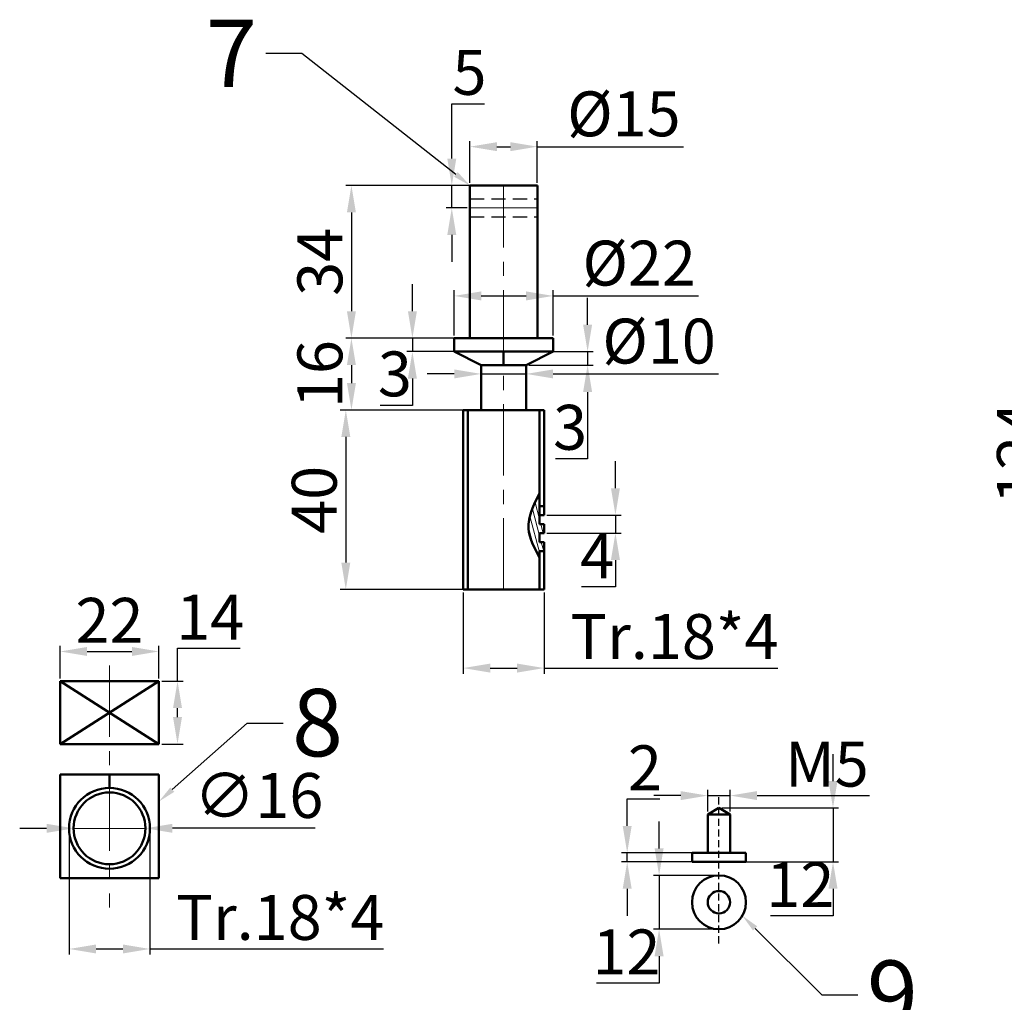
# Model space of a CAD drawing. Units: millimetres. Extents: x 147 to 984, y -369 to 435.
# Tile 6 of 10: x 480 to 699, y -48 to 171. Entities that reach past the tile are written whole.
import ezdxf
from ezdxf import colors
from ezdxf.entities.mleader import LeaderData, LeaderLine
from ezdxf.math import Vec2, Vec3

# ---------------------------------------------------------------- set-up
doc = ezdxf.new("R2010")
doc.units = ezdxf.units.MM
doc.header["$LTSCALE"] = 0.5
doc.linetypes.add('CENTER', pattern=[50.8, 31.75, -6.35, 6.35, -6.35])
doc.linetypes.add('HIDDEN', pattern=[9.525, 6.35, -3.175])
for name, color, linetype, lineweight in [('M-CNTR', 1, 'CENTER', 18), ('M-DIMS', 2, 'Continuous', 25), ('M-HATC', 8, 'Continuous', 18), ('M-HIDN', 3, 'HIDDEN', 25), ('M-OUTL', 7, 'Continuous', 50), ('M-TEXT', 7, 'Continuous', 25)]:
    doc.layers.add(name, color=color, linetype=linetype, lineweight=lineweight)
doc.styles.get("Standard").update_dxf_attribs({"font": 'arial.ttf'})
doc.dimstyles.new('ISO-25', dxfattribs={"dimtxt": 10, "dimasz": 6, "dimexe": 1.25, "dimexo": 0.625, "dimtad": 1, "dimtoh": 1, "dimdec": 0, "dimtxsty": 'Standard', "dimcen": 2.5, "dimadec": 0, "dimazin": 0, "dimtfac": 1, "dimtdec": 0, "dimtmove": 0, "dimatfit": 3, "dimfxl": 1, "dimarcsym": 0})

# ---------------------------------------------------------------- blocks, each defined once
blk = doc.blocks.new('*D63')
at = {"layer": 'Defpoints', "color": 0, "transparency": 16777216}
for p in [(800.56, 136.03), (709.78, 12.03), (800.56, 12.03)]:
    blk.add_point(p, dxfattribs=at)
at = {"layer": 'M-DIMS', "color": 0, "lineweight": -2, "transparency": 16777216}
for p, q in [((799.93, 136.03), (708.53, 136.03)), ((709.78, 130.03), (709.78, 18.03)), ((799.93, 12.03), (708.53, 12.03))]:
    blk.add_line(p, q, dxfattribs=at)
at = {"layer": 'M-DIMS', "color": 0, "transparency": 16777216}
for points in [[(708.78, 130.03), (710.78, 130.03), (709.78, 136.03)], [(708.78, 18.03), (710.78, 18.03), (709.78, 12.03)]]:
    blk.add_solid(points, dxfattribs=at)
at = {"layer": 'M-DIMS', "color": 0, "transparency": 16777216, "insert": (704.14, 74.03), "char_height": 10, "attachment_point": 5, "rotation": 90}
blk.add_mtext('124', dxfattribs=at)
blk = doc.blocks.new('*D75')
at = {"layer": 'Defpoints', "color": 0, "ltscale": 0.5, "transparency": 16777216}
for p in [(595.48, 142.24), (580.48, 133.59), (595.48, 133.59)]:
    blk.add_point(p, dxfattribs=at)
at = {"layer": 'M-DIMS', "color": 0, "lineweight": -2, "ltscale": 0.5, "transparency": 16777216}
for p, q in [((580.48, 134.22), (580.48, 143.49)), ((595.48, 134.22), (595.48, 143.49)), ((586.48, 142.24), (589.48, 142.24)), ((595.48, 142.24), (628.01, 142.24))]:
    blk.add_line(p, q, dxfattribs=at)
at = {"layer": 'M-DIMS', "color": 0, "ltscale": 0.5, "transparency": 16777216}
for points in [[(586.48, 143.24), (586.48, 141.24), (580.48, 142.24)], [(589.48, 143.24), (589.48, 141.24), (595.48, 142.24)]]:
    blk.add_solid(points, dxfattribs=at)
at = {"layer": 'M-DIMS', "color": 0, "ltscale": 0.5, "transparency": 16777216, "insert": (614.75, 148.25), "char_height": 10, "attachment_point": 5}
blk.add_mtext('%%C15', dxfattribs=at)
blk = doc.blocks.new('*D76')
at = {"layer": 'Defpoints', "color": 0, "ltscale": 0.5, "transparency": 16777216}
for p in [(580.48, 133.59), (576.43, 128.59), (580.48, 128.59)]:
    blk.add_point(p, dxfattribs=at)
at = {"layer": 'M-DIMS', "color": 0, "lineweight": -2, "ltscale": 0.5, "transparency": 16777216}
for p, q in [((576.43, 139.59), (576.43, 151.78)), ((576.43, 151.78), (583.68, 151.78)), ((579.86, 133.59), (575.18, 133.59)), ((576.43, 128.59), (576.43, 133.59)), ((579.86, 128.59), (575.18, 128.59)), ((576.43, 122.59), (576.43, 116.59))]:
    blk.add_line(p, q, dxfattribs=at)
at = {"layer": 'M-DIMS', "color": 0, "ltscale": 0.5, "transparency": 16777216}
for points in [[(575.43, 139.59), (577.43, 139.59), (576.43, 133.59)], [(575.43, 122.59), (577.43, 122.59), (576.43, 128.59)]]:
    blk.add_solid(points, dxfattribs=at)
at = {"layer": 'M-DIMS', "color": 0, "ltscale": 0.5, "transparency": 16777216, "insert": (580.37, 157.49), "char_height": 10, "attachment_point": 5}
blk.add_mtext('5', dxfattribs=at)
blk = doc.blocks.new('*D77')
at = {"layer": 'Defpoints', "color": 0, "ltscale": 0.5, "transparency": 16777216}
for p in [(587.98, 133.59), (554.08, 99.59), (587.98, 99.59)]:
    blk.add_point(p, dxfattribs=at)
at = {"layer": 'M-DIMS', "color": 0, "lineweight": -2, "ltscale": 0.5, "transparency": 16777216}
for p, q in [((587.36, 133.59), (552.83, 133.59)), ((554.08, 127.59), (554.08, 105.59)), ((587.36, 99.59), (552.83, 99.59))]:
    blk.add_line(p, q, dxfattribs=at)
at = {"layer": 'M-DIMS', "color": 0, "ltscale": 0.5, "transparency": 16777216}
for points in [[(553.08, 127.59), (555.08, 127.59), (554.08, 133.59)], [(553.08, 105.59), (555.08, 105.59), (554.08, 99.59)]]:
    blk.add_solid(points, dxfattribs=at)
at = {"layer": 'M-DIMS', "color": 0, "ltscale": 0.5, "transparency": 16777216, "insert": (548.35, 116.59), "char_height": 10, "attachment_point": 5, "rotation": 90}
blk.add_mtext('34', dxfattribs=at)
blk = doc.blocks.new('*D78')
at = {"layer": 'Defpoints', "color": 0, "ltscale": 0.5, "transparency": 16777216}
for p in [(587.98, 99.59), (554.08, 83.59), (587.98, 83.59)]:
    blk.add_point(p, dxfattribs=at)
at = {"layer": 'M-DIMS', "color": 0, "lineweight": -2, "ltscale": 0.5, "transparency": 16777216}
for p, q in [((587.36, 99.59), (552.83, 99.59)), ((554.08, 93.59), (554.08, 89.59)), ((587.36, 83.59), (552.83, 83.59))]:
    blk.add_line(p, q, dxfattribs=at)
at = {"layer": 'M-DIMS', "color": 0, "ltscale": 0.5, "transparency": 16777216}
for points in [[(553.08, 93.59), (555.08, 93.59), (554.08, 99.59)], [(553.08, 89.59), (555.08, 89.59), (554.08, 83.59)]]:
    blk.add_solid(points, dxfattribs=at)
at = {"layer": 'M-DIMS', "color": 0, "ltscale": 0.5, "transparency": 16777216, "insert": (548.35, 91.59), "char_height": 10, "attachment_point": 5, "rotation": 90}
blk.add_mtext('16', dxfattribs=at)
blk = doc.blocks.new('*D79')
at = {"layer": 'Defpoints', "color": 0, "ltscale": 0.5, "transparency": 16777216}
for p in [(587.98, 83.59), (552.83, 43.59), (587.98, 43.59)]:
    blk.add_point(p, dxfattribs=at)
at = {"layer": 'M-DIMS', "color": 0, "lineweight": -2, "ltscale": 0.5, "transparency": 16777216}
for p, q in [((587.36, 83.59), (551.58, 83.59)), ((552.83, 77.59), (552.83, 49.59)), ((587.36, 43.59), (551.58, 43.59))]:
    blk.add_line(p, q, dxfattribs=at)
at = {"layer": 'M-DIMS', "color": 0, "ltscale": 0.5, "transparency": 16777216}
for points in [[(551.83, 77.59), (553.83, 77.59), (552.83, 83.59)], [(551.83, 49.59), (553.83, 49.59), (552.83, 43.59)]]:
    blk.add_solid(points, dxfattribs=at)
at = {"layer": 'M-DIMS', "color": 0, "ltscale": 0.5, "transparency": 16777216, "insert": (547.1, 63.59), "char_height": 10, "attachment_point": 5, "rotation": 90}
blk.add_mtext('40', dxfattribs=at)
blk = doc.blocks.new('*D80')
at = {"layer": 'Defpoints', "color": 0, "ltscale": 0.5, "transparency": 16777216}
for p in [(592.98, 91.63), (582.98, 88.59), (592.98, 88.59)]:
    blk.add_point(p, dxfattribs=at)
at = {"layer": 'M-DIMS', "color": 0, "lineweight": -2, "ltscale": 0.5, "transparency": 16777216}
for p, q in [((582.98, 89.22), (582.98, 92.88)), ((592.98, 89.22), (592.98, 92.88)), ((576.98, 91.63), (570.98, 91.63)), ((582.98, 91.63), (592.98, 91.63)), ((598.98, 91.63), (635.81, 91.63))]:
    blk.add_line(p, q, dxfattribs=at)
at = {"layer": 'M-DIMS', "color": 0, "ltscale": 0.5, "transparency": 16777216}
for points in [[(576.98, 92.63), (576.98, 90.63), (582.98, 91.63)], [(598.98, 92.63), (598.98, 90.63), (592.98, 91.63)]]:
    blk.add_solid(points, dxfattribs=at)
at = {"layer": 'M-DIMS', "color": 0, "ltscale": 0.5, "transparency": 16777216, "insert": (622.6, 97.64), "char_height": 10, "attachment_point": 5}
blk.add_mtext('%%C10', dxfattribs=at)
blk = doc.blocks.new('*D81')
at = {"layer": 'Defpoints', "color": 0, "ltscale": 0.5, "transparency": 16777216}
for p in [(598.98, 109), (576.98, 99.59), (598.98, 99.59)]:
    blk.add_point(p, dxfattribs=at)
at = {"layer": 'M-DIMS', "color": 0, "lineweight": -2, "ltscale": 0.5, "transparency": 16777216}
for p, q in [((576.98, 100.22), (576.98, 110.25)), ((598.98, 100.22), (598.98, 110.25)), ((582.98, 109), (592.98, 109)), ((598.98, 109), (631.34, 109))]:
    blk.add_line(p, q, dxfattribs=at)
at = {"layer": 'M-DIMS', "color": 0, "ltscale": 0.5, "transparency": 16777216}
for points in [[(582.98, 110), (582.98, 108), (576.98, 109)], [(592.98, 110), (592.98, 108), (598.98, 109)]]:
    blk.add_solid(points, dxfattribs=at)
at = {"layer": 'M-DIMS', "color": 0, "ltscale": 0.5, "transparency": 16777216, "insert": (618.16, 115.01), "char_height": 10, "attachment_point": 5}
blk.add_mtext('%%C22', dxfattribs=at)
blk = doc.blocks.new('*D82')
at = {"layer": 'Defpoints', "color": 0, "ltscale": 0.5, "transparency": 16777216}
for p in [(587.98, 99.59), (567.66, 96.59), (587.98, 96.59)]:
    blk.add_point(p, dxfattribs=at)
at = {"layer": 'M-DIMS', "color": 0, "lineweight": -2, "ltscale": 0.5, "transparency": 16777216}
for p, q in [((567.66, 105.59), (567.66, 111.59)), ((587.36, 99.59), (566.41, 99.59)), ((567.66, 99.59), (567.66, 96.59)), ((587.36, 96.59), (566.41, 96.59)), ((567.66, 90.59), (567.66, 84.59)), ((567.66, 84.59), (560.49, 84.59))]:
    blk.add_line(p, q, dxfattribs=at)
at = {"layer": 'M-DIMS', "color": 0, "ltscale": 0.5, "transparency": 16777216}
for points in [[(566.66, 105.59), (568.66, 105.59), (567.66, 99.59)], [(566.66, 90.59), (568.66, 90.59), (567.66, 96.59)]]:
    blk.add_solid(points, dxfattribs=at)
at = {"layer": 'M-DIMS', "color": 0, "ltscale": 0.5, "transparency": 16777216, "insert": (563.76, 90.33), "char_height": 10, "attachment_point": 5}
blk.add_mtext('3', dxfattribs=at)
blk = doc.blocks.new('*D83')
at = {"layer": 'Defpoints', "color": 0, "ltscale": 0.5, "transparency": 16777216}
for p in [(592.98, 96.59), (606.68, 96.59), (592.98, 93.59)]:
    blk.add_point(p, dxfattribs=at)
at = {"layer": 'M-DIMS', "color": 0, "lineweight": -2, "ltscale": 0.5, "transparency": 16777216}
for p, q in [((606.68, 102.59), (606.68, 108.59)), ((593.61, 96.59), (607.93, 96.59)), ((606.68, 96.59), (606.68, 93.59)), ((593.61, 93.59), (607.93, 93.59)), ((606.68, 87.59), (606.68, 72.7)), ((606.68, 72.7), (599.5, 72.7))]:
    blk.add_line(p, q, dxfattribs=at)
at = {"layer": 'M-DIMS', "color": 0, "ltscale": 0.5, "transparency": 16777216}
for points in [[(605.68, 102.59), (607.68, 102.59), (606.68, 96.59)], [(605.68, 87.59), (607.68, 87.59), (606.68, 93.59)]]:
    blk.add_solid(points, dxfattribs=at)
at = {"layer": 'M-DIMS', "color": 0, "ltscale": 0.5, "transparency": 16777216, "insert": (602.78, 78.44), "char_height": 10, "attachment_point": 5}
blk.add_mtext('3', dxfattribs=at)
blk = doc.blocks.new('*D84')
at = {"layer": 'Defpoints', "color": 0, "ltscale": 0.5, "transparency": 16777216}
for p in [(596.98, 60.18), (596.98, 56.18), (612.88, 56.18)]:
    blk.add_point(p, dxfattribs=at)
at = {"layer": 'M-DIMS', "color": 0, "lineweight": -2, "ltscale": 0.5, "transparency": 16777216}
for p, q in [((612.88, 66.18), (612.88, 72.18)), ((597.61, 60.18), (614.13, 60.18)), ((612.88, 60.18), (612.88, 56.18)), ((597.61, 56.18), (614.13, 56.18)), ((612.88, 50.18), (612.88, 44.18)), ((612.88, 44.18), (605.34, 44.18))]:
    blk.add_line(p, q, dxfattribs=at)
at = {"layer": 'M-DIMS', "color": 0, "ltscale": 0.5, "transparency": 16777216}
for points in [[(611.88, 66.18), (613.88, 66.18), (612.88, 60.18)], [(611.88, 50.18), (613.88, 50.18), (612.88, 56.18)]]:
    blk.add_solid(points, dxfattribs=at)
at = {"layer": 'M-DIMS', "color": 0, "ltscale": 0.5, "transparency": 16777216, "insert": (608.8, 49.81), "char_height": 10, "attachment_point": 5}
blk.add_mtext('4', dxfattribs=at)
blk = doc.blocks.new('*D85')
at = {"layer": 'Defpoints', "color": 0, "ltscale": 0.5, "transparency": 16777216}
for p in [(578.98, 43.59), (596.98, 43.59), (596.98, 26.11)]:
    blk.add_point(p, dxfattribs=at)
at = {"layer": 'M-DIMS', "color": 0, "lineweight": -2, "ltscale": 0.5, "transparency": 16777216}
for p, q in [((578.98, 42.97), (578.98, 24.86)), ((596.98, 42.97), (596.98, 24.86)), ((584.98, 26.11), (590.98, 26.11)), ((596.98, 26.11), (649.04, 26.11))]:
    blk.add_line(p, q, dxfattribs=at)
at = {"layer": 'M-DIMS', "color": 0, "ltscale": 0.5, "transparency": 16777216}
for points in [[(584.98, 27.11), (584.98, 25.11), (578.98, 26.11)], [(590.98, 27.11), (590.98, 25.11), (596.98, 26.11)]]:
    blk.add_solid(points, dxfattribs=at)
at = {"layer": 'M-DIMS', "color": 0, "ltscale": 0.5, "transparency": 16777216, "insert": (626.01, 31.84), "char_height": 10, "attachment_point": 5}
blk.add_mtext('Tr.18*4', dxfattribs=at)
blk = doc.blocks.new('*U86')
at = {"layer": 'M-CNTR', "color": 0, "transparency": 16777216}
blk.add_line((0, 10.5), (0, -43.39), dxfattribs=at)
blk = doc.blocks.new('*D87')
at = {"layer": 'Defpoints', "color": 0, "ltscale": 0.5, "transparency": 16777216}
for p in [(491.2, -9.58), (509.2, -9.58), (509.2, -36.45)]:
    blk.add_point(p, dxfattribs=at)
at = {"layer": 'M-DIMS', "color": 0, "lineweight": -2, "ltscale": 0.5, "transparency": 16777216}
for p, q in [((491.2, -10.2), (491.2, -37.7)), ((509.2, -10.2), (509.2, -37.7)), ((497.2, -36.45), (503.2, -36.45)), ((509.2, -36.45), (561.26, -36.45))]:
    blk.add_line(p, q, dxfattribs=at)
at = {"layer": 'M-DIMS', "color": 0, "ltscale": 0.5, "transparency": 16777216}
for points in [[(497.2, -35.45), (497.2, -37.45), (491.2, -36.45)], [(503.2, -35.45), (503.2, -37.45), (509.2, -36.45)]]:
    blk.add_solid(points, dxfattribs=at)
at = {"layer": 'M-DIMS', "color": 0, "ltscale": 0.5, "transparency": 16777216, "insert": (538.23, -30.72), "char_height": 10, "attachment_point": 5}
blk.add_mtext('Tr.18*4', dxfattribs=at)
blk = doc.blocks.new('*D88')
at = {"layer": 'Defpoints', "color": 0, "ltscale": 0.5, "transparency": 16777216}
for p in [(511.2, 23.19), (511.2, 9.19), (515.35, 9.19)]:
    blk.add_point(p, dxfattribs=at)
at = {"layer": 'M-DIMS', "color": 0, "lineweight": -2, "ltscale": 0.5, "transparency": 16777216}
for p, q in [((515.35, 23.19), (515.35, 30.52)), ((515.35, 30.52), (529.31, 30.52)), ((511.83, 23.19), (516.6, 23.19)), ((515.35, 15.19), (515.35, 17.19)), ((511.83, 9.19), (516.6, 9.19))]:
    blk.add_line(p, q, dxfattribs=at)
at = {"layer": 'M-DIMS', "color": 0, "ltscale": 0.5, "transparency": 16777216}
for points in [[(514.35, 17.19), (516.35, 17.19), (515.35, 23.19)], [(514.35, 15.19), (516.35, 15.19), (515.35, 9.19)]]:
    blk.add_solid(points, dxfattribs=at)
at = {"layer": 'M-DIMS', "color": 0, "ltscale": 0.5, "transparency": 16777216, "insert": (522.64, 36.17), "char_height": 10, "attachment_point": 5}
blk.add_mtext('14', dxfattribs=at)
blk = doc.blocks.new('*D89')
at = {"layer": 'Defpoints', "color": 0, "ltscale": 0.5, "transparency": 16777216}
for p in [(511.2, 29.81), (489.2, 23.19), (511.2, 23.19)]:
    blk.add_point(p, dxfattribs=at)
at = {"layer": 'M-DIMS', "color": 0, "lineweight": -2, "ltscale": 0.5, "transparency": 16777216}
for p, q in [((489.2, 23.81), (489.2, 31.06)), ((511.2, 23.81), (511.2, 31.06)), ((495.2, 29.81), (505.2, 29.81))]:
    blk.add_line(p, q, dxfattribs=at)
at = {"layer": 'M-DIMS', "color": 0, "ltscale": 0.5, "transparency": 16777216}
for points in [[(495.2, 30.81), (495.2, 28.81), (489.2, 29.81)], [(505.2, 30.81), (505.2, 28.81), (511.2, 29.81)]]:
    blk.add_solid(points, dxfattribs=at)
at = {"layer": 'M-DIMS', "color": 0, "ltscale": 0.5, "transparency": 16777216, "insert": (500.2, 35.45), "char_height": 10, "attachment_point": 5}
blk.add_mtext('22', dxfattribs=at)
blk = doc.blocks.new('*D90')
at = {"layer": 'Defpoints', "color": 0, "ltscale": 0.5, "transparency": 16777216}
for p in [(635.93, -20.05), (622.6, -32.05), (635.93, -32.05)]:
    blk.add_point(p, dxfattribs=at)
at = {"layer": 'M-DIMS', "color": 0, "lineweight": -2, "ltscale": 0.5, "transparency": 16777216}
for p, q in [((622.6, -14.05), (622.6, -8.05)), ((635.31, -20.05), (621.35, -20.05)), ((622.6, -20.05), (622.6, -32.05)), ((635.31, -32.05), (621.35, -32.05)), ((622.6, -38.05), (622.6, -44.05)), ((622.6, -44.05), (608.69, -44.05))]:
    blk.add_line(p, q, dxfattribs=at)
at = {"layer": 'M-DIMS', "color": 0, "ltscale": 0.5, "transparency": 16777216}
for points in [[(621.6, -14.05), (623.6, -14.05), (622.6, -20.05)], [(621.6, -38.05), (623.6, -38.05), (622.6, -32.05)]]:
    blk.add_solid(points, dxfattribs=at)
at = {"layer": 'M-DIMS', "color": 0, "ltscale": 0.5, "transparency": 16777216, "insert": (615.33, -38.4), "char_height": 10, "attachment_point": 5}
blk.add_mtext('12', dxfattribs=at)
blk = doc.blocks.new('*D91')
at = {"layer": 'Defpoints', "color": 0, "ltscale": 0.5, "transparency": 16777216}
for p in [(638.43, -2.29), (633.43, -6.48), (638.43, -6.48)]:
    blk.add_point(p, dxfattribs=at)
at = {"layer": 'M-DIMS', "color": 0, "lineweight": -2, "ltscale": 0.5, "transparency": 16777216}
for p, q in [((633.43, -5.86), (633.43, -1.04)), ((638.43, -5.86), (638.43, -1.04)), ((627.43, -2.29), (621.43, -2.29)), ((633.43, -2.29), (638.43, -2.29)), ((644.43, -2.29), (669.49, -2.29))]:
    blk.add_line(p, q, dxfattribs=at)
at = {"layer": 'M-DIMS', "color": 0, "ltscale": 0.5, "transparency": 16777216}
for points in [[(627.43, -1.29), (627.43, -3.29), (633.43, -2.29)], [(644.43, -1.29), (644.43, -3.29), (638.43, -2.29)]]:
    blk.add_solid(points, dxfattribs=at)
at = {"layer": 'M-DIMS', "color": 0, "ltscale": 0.5, "transparency": 16777216, "insert": (659.96, 3.42), "char_height": 10, "attachment_point": 5}
blk.add_mtext('M5', dxfattribs=at)
blk = doc.blocks.new('*D92')
at = {"layer": 'Defpoints', "color": 0, "ltscale": 0.5, "transparency": 16777216}
for p in [(635.93, -5.04), (635.93, -17.04), (661.33, -17.04)]:
    blk.add_point(p, dxfattribs=at)
at = {"layer": 'M-DIMS', "color": 0, "lineweight": -2, "ltscale": 0.5, "transparency": 16777216}
for p, q in [((661.33, 0.96), (661.33, 6.96)), ((636.56, -5.04), (662.58, -5.04)), ((661.33, -5.04), (661.33, -17.04)), ((636.56, -17.04), (662.58, -17.04)), ((661.33, -23.04), (661.33, -29.04)), ((661.33, -29.04), (647.43, -29.04))]:
    blk.add_line(p, q, dxfattribs=at)
at = {"layer": 'M-DIMS', "color": 0, "ltscale": 0.5, "transparency": 16777216}
for points in [[(660.33, 0.96), (662.33, 0.96), (661.33, -5.04)], [(660.33, -23.04), (662.33, -23.04), (661.33, -17.04)]]:
    blk.add_solid(points, dxfattribs=at)
at = {"layer": 'M-DIMS', "color": 0, "ltscale": 0.5, "transparency": 16777216, "insert": (654.07, -23.39), "char_height": 10, "attachment_point": 5}
blk.add_mtext('12', dxfattribs=at)
blk = doc.blocks.new('*D93')
at = {"layer": 'Defpoints', "color": 0, "ltscale": 0.5, "transparency": 16777216}
for p in [(641.93, -15.04), (615.5, -17.04), (641.93, -17.04)]:
    blk.add_point(p, dxfattribs=at)
at = {"layer": 'M-DIMS', "color": 0, "lineweight": -2, "ltscale": 0.5, "transparency": 16777216}
for p, q in [((615.5, -9.04), (615.5, -3.04)), ((615.5, -3.04), (622.75, -3.04)), ((641.31, -15.04), (614.25, -15.04)), ((615.5, -17.04), (615.5, -15.04)), ((641.31, -17.04), (614.25, -17.04)), ((615.5, -23.04), (615.5, -29.04))]:
    blk.add_line(p, q, dxfattribs=at)
at = {"layer": 'M-DIMS', "color": 0, "ltscale": 0.5, "transparency": 16777216}
for points in [[(614.5, -9.04), (616.5, -9.04), (615.5, -15.04)], [(614.5, -23.04), (616.5, -23.04), (615.5, -17.04)]]:
    blk.add_solid(points, dxfattribs=at)
at = {"layer": 'M-DIMS', "color": 0, "ltscale": 0.5, "transparency": 16777216, "insert": (619.44, 2.61), "char_height": 10, "attachment_point": 5}
blk.add_mtext('2', dxfattribs=at)
blk = doc.blocks.new('*D192')
at = {"layer": 'Defpoints', "color": 0, "ltscale": 0.5, "transparency": 16777216}
for p in [(492.2, -9.58), (508.2, -9.57)]:
    blk.add_point(p, dxfattribs=at)
at = {"layer": 'M-DIMS', "color": 0, "lineweight": -2, "ltscale": 0.5, "transparency": 16777216}
for p, q in [((486.2, -9.58), (480.2, -9.58)), ((492.2, -9.58), (508.2, -9.57)), ((520.2, -9.57), (514.2, -9.57)), ((546.02, -9.57), (520.2, -9.57))]:
    blk.add_line(p, q, dxfattribs=at)
at = {"layer": 'M-DIMS', "color": 0, "ltscale": 0.5, "transparency": 16777216}
for points in [[(486.2, -8.58), (486.2, -10.58), (492.2, -9.58)], [(514.2, -8.57), (514.2, -10.57), (508.2, -9.57)]]:
    blk.add_solid(points, dxfattribs=at)
at = {"layer": 'M-DIMS', "color": 0, "ltscale": 0.5, "transparency": 16777216, "insert": (533.43, -3.56), "char_height": 10, "attachment_point": 5}
blk.add_mtext('∅16', dxfattribs=at)

msp = doc.modelspace()

# ---------------------------------------------------------------- hatches: boundary and pattern name
at = {"layer": 'M-HATC', "ltscale": 0.5}
h = msp.add_hatch(dxfattribs=at)
h.set_pattern_fill('ANSI31', color=256, scale=0.3, angle=60)
h.set_pattern_definition([(105, (388.46085, 296.464), (-0.9200443, -0.246525), [])])
edge = h.paths.add_edge_path()
edge.add_line((595.9849, 56.1829), (596.9849, 56.1829))
edge.add_line((596.9849, 56.1829), (596.9849, 58.1829))
edge.add_line((596.9849, 58.1829), (595.9849, 58.1829))
edge.add_line((595.9849, 58.1829), (595.9849, 60.1829))
edge.add_line((595.9849, 60.1829), (595.9849, 65.0785))
edge.add_spline(control_points=[(595.9849, 65.0785), (594.6742, 62.4476), (592.2595, 57.6008), (594.8161, 52.9018), (595.9849, 50.7535)], knot_values=[0, 0, 0, 0, 8.22780848, 15.15780962, 15.15780962, 15.15780962, 15.15780962], degree=3, periodic=0)
edge.add_line((595.9849, 50.7535), (595.9849, 52.1829))
edge.add_line((595.9849, 52.1829), (596.9849, 52.1829))
edge.add_line((596.9849, 52.1829), (596.9849, 54.1829))
edge.add_line((596.9849, 54.1829), (595.9849, 54.1829))
edge.add_line((595.9849, 54.1829), (595.9849, 56.1829))

# ---------------------------------------------------------------- linework, layer by layer
at = {"layer": 'M-CNTR'}
for p, q in [((587.9849, 43.5911), (587.9849, 133.5911)), ((580.4849, 128.5911), (595.4849, 128.5911))]:
    msp.add_line(p, q, dxfattribs=at)
at = {"layer": 'M-HIDN'}
for p, q in [((580.4849, 130.5911), (595.4849, 130.5911)), ((580.4849, 126.5911), (595.4849, 126.5911))]:
    msp.add_line(p, q, dxfattribs=at)
at = {"layer": 'M-HIDN', "ltscale": 0.5}
msp.add_line((635.9344, -35.2113), (635.9344, -2.2979), dxfattribs=at)
at = {"layer": 'M-OUTL'}
for p, q in [((580.4849, 133.5911), (595.4849, 133.5911)), ((580.4849, 133.5911), (580.4849, 99.5911)), ((595.4849, 133.5911), (595.4849, 99.5911)), ((576.9849, 99.5911), (598.9849, 99.5911)), ((576.9849, 96.5911), (576.9849, 99.5911)), ((598.9849, 99.5911), (598.9849, 96.5911)), ((598.9849, 96.5911), (576.9849, 96.5911)), ((582.9849, 93.5911), (576.9849, 96.5911)), ((587.9849, 96.5911), (587.9849, 93.5911)), ((592.9849, 93.5911), (598.9849, 96.5911)), ((592.9849, 93.5911), (582.9849, 93.5911)), ((582.9849, 93.5911), (582.9849, 83.5911)), ((592.9849, 83.5911), (592.9849, 93.5911)), ((596.9849, 83.5911), (578.9849, 83.5911)), ((578.9849, 83.5911), (578.9849, 43.5911)), ((579.9849, 83.5911), (579.9849, 43.5911)), ((582.9849, 83.5911), (592.9849, 83.5911)), ((595.9849, 58.1829), (595.9849, 83.5911)), ((596.9849, 60.1829), (596.9849, 83.5911)), ((596.9849, 56.1829), (596.9849, 58.1829)), ((595.9849, 54.1829), (595.9849, 56.1829)), ((596.9849, 43.5911), (596.9849, 54.1829)), ((595.9849, 43.5911), (595.9849, 52.1829)), ((578.9849, 43.5911), (596.9849, 43.5911))]:
    msp.add_line(p, q, dxfattribs=at)
at = {"layer": 'M-OUTL', "ltscale": 0.5}
for p, q in [((595.9849, 62.1829), (596.9849, 62.1829)), ((596.9849, 60.1829), (595.9849, 60.1829)), ((595.9849, 60.1829), (595.9849, 58.1829)), ((595.9849, 58.1829), (596.9849, 58.1829)), ((596.9849, 58.1829), (596.9849, 56.1829)), ((596.9849, 56.1829), (595.9849, 56.1829)), ((595.9849, 56.1829), (595.9849, 54.1829)), ((595.9849, 54.1829), (596.9849, 54.1829)), ((596.9849, 54.1829), (596.9849, 52.1829)), ((596.9849, 52.1829), (595.9849, 52.1829)), ((489.2017, 23.1877), (511.2017, 23.1877)), ((489.2017, 9.1877), (489.2017, 23.1877)), ((489.2017, 23.1877), (511.2017, 9.1877)), ((511.2017, 23.1877), (489.2017, 9.1877)), ((511.2017, 23.1877), (511.2017, 9.1877)), ((511.2017, 9.1877), (489.2017, 9.1877)), ((489.2017, 2.4246), (489.2017, -20.7067)), ((500.2017, 2.4246), (489.2017, 2.4246)), ((500.2017, -0.5754), (500.2017, 2.4246)), ((500.2017, 2.4246), (511.2017, 2.4246)), ((511.2017, 2.4246), (511.2017, -20.7067)), ((635.9344, -5.0372), (633.4344, -6.4805)), ((633.4344, -6.4805), (633.4344, -15.0372)), ((633.4344, -6.4805), (638.4344, -6.4805)), ((635.9344, -5.0372), (638.4344, -6.4805)), ((638.4344, -6.4805), (638.4344, -15.0372)), ((641.9344, -15.0372), (629.9344, -15.0372)), ((629.9344, -15.0372), (629.9344, -17.0372)), ((641.9344, -17.0372), (641.9344, -15.0372)), ((629.9344, -17.0372), (641.9344, -17.0372)), ((489.2017, -20.7067), (511.2017, -20.7067))]:
    msp.add_line(p, q, dxfattribs=at)
for centre, radius in [((500.2017, -9.5754), 9), ((500.2017, -9.5754), 8), ((635.9344, -26.0481), 6), ((635.9344, -26.0481), 2.5)]:
    msp.add_circle(centre, radius, dxfattribs=at)
msp.add_open_spline([(595.9849, 65.0785), (594.6742, 62.4476), (592.2595, 57.6008), (594.8161, 52.9018), (595.9849, 50.7535)], degree=3, knots=[0, 0, 0, 0, 8.22780848, 15.15780962, 15.15780962, 15.15780962, 15.15780962], dxfattribs=at)

# ---------------------------------------------------------------- block references
at = {"layer": 'M-CNTR'}
msp.add_blockref('*U86', (500.2017, 16.1877), dxfattribs=at)

# ---------------------------------------------------------------- dimensions: what is measured, and where the dimension line sits
at = {"layer": 'M-DIMS', "ltscale": 0.5}
for base, p1, p2, picture, middle in [((576.4279, 128.5911), (580.4849, 133.5911), (580.4849, 128.5911), '*D76', (580.3681, 151.7786)), ((606.6772, 96.5911), (592.9849, 93.5911), (592.9849, 96.5911), '*D83', (602.778, 72.7029)), ((515.346, 9.1877), (511.2017, 23.1877), (511.2017, 9.1877), '*D88', (522.6423, 30.523)), ((615.5042, -17.0372), (641.9344, -15.0372), (641.9344, -17.0372), '*D93', (619.4409, -3.0372))]:
    dim = msp.add_linear_dim(base=base, p1=p1, p2=p2, angle=90, dimstyle='ISO-25', override={"dimclrd": 0, "dimclre": 0, "dimclrt": 0}, dxfattribs=at)
    dim.commit()
    dim.dimension.update_dxf_attribs({"geometry": picture, "text_midpoint": middle, "dimtype": 160})
for base, p1, p2, text, picture, middle in [((595.4849, 142.2366), (580.4849, 133.5911), (595.4849, 133.5911), '%%C<>', '*D75', (614.7498, 148.247)), ((598.9849, 109.0014), (576.9849, 99.5911), (598.9849, 99.5911), '%%C<>', '*D81', (618.1611, 115.0118)), ((596.9849, 26.1114), (578.9849, 43.5911), (596.9849, 43.5911), 'Tr.<>*4', '*D85', (626.0144, 31.8421)), ((638.4344, -2.2907), (633.4344, -6.4805), (638.4344, -6.4805), 'M<>', '*D91', (659.9646, 3.4196)), ((509.2017, -36.4532), (491.2017, -9.5754), (509.2017, -9.5754), 'Tr.<>*4', '*D87', (538.2312, -30.7225))]:
    dim = msp.add_linear_dim(base=base, p1=p1, p2=p2, text=text, dimstyle='ISO-25', override={"dimclrd": 0, "dimclre": 0, "dimclrt": 0}, dxfattribs=at)
    dim.commit()
    dim.dimension.update_dxf_attribs({"geometry": picture, "text_midpoint": middle})
at = {"layer": 'M-DIMS'}
dim = msp.add_linear_dim(base=(709.7842, 12.0279), p1=(800.5575, 136.0279), p2=(800.5575, 12.0279), angle=90, dimstyle='ISO-25', override={"dimclrd": 0, "dimclre": 0, "dimclrt": 0}, dxfattribs=at)
dim.commit()
dim.dimension.update_dxf_attribs({"geometry": '*D63', "text_midpoint": (704.1387, 74.0279)})
at = {"layer": 'M-DIMS', "ltscale": 0.5}
for base, p1, p2, picture, middle in [((554.0806, 99.5911), (587.9849, 133.5911), (587.9849, 99.5911), '*D77', (548.3465, 116.5911)), ((567.6592, 96.5911), (587.9849, 99.5911), (587.9849, 96.5911), '*D82', (563.7599, 90.3252)), ((554.0806, 83.5911), (587.9849, 99.5911), (587.9849, 83.5911), '*D78', (548.3499, 91.5911)), ((552.8306, 43.5911), (587.9849, 83.5911), (587.9849, 43.5911), '*D79', (547.0999, 63.5911)), ((612.8842, 56.1829), (596.9849, 60.1829), (596.9849, 56.1829), '*D84', (608.8008, 49.8079)), ((661.3323, -17.0372), (635.9344, -5.0372), (635.9344, -17.0372), '*D92', (654.0668, -23.3917)), ((622.5955, -32.0481), (635.9344, -20.0481), (635.9344, -32.0481), '*D90', (615.33, -38.4027))]:
    dim = msp.add_linear_dim(base=base, p1=p1, p2=p2, angle=90, dimstyle='ISO-25', override={"dimclrd": 0, "dimclre": 0, "dimclrt": 0}, dxfattribs=at)
    dim.commit()
    dim.dimension.update_dxf_attribs({"geometry": picture, "text_midpoint": middle})
dim = msp.add_linear_dim(base=(592.9849, 91.6325), p1=(582.9849, 88.5911), p2=(592.9849, 88.5911), text='%%C<>', dimstyle='ISO-25', override={"dimclrd": 0, "dimclre": 0, "dimclrt": 0}, dxfattribs=at)
dim.commit()
dim.dimension.update_dxf_attribs({"geometry": '*D80', "text_midpoint": (622.6006, 91.6325), "dimtype": 160})
dim = msp.add_linear_dim(base=(511.2017, 29.8094), p1=(489.2017, 23.1877), p2=(511.2017, 23.1877), dimstyle='ISO-25', override={"dimclrd": 0, "dimclre": 0, "dimclrt": 0}, dxfattribs=at)
dim.commit()
dim.dimension.update_dxf_attribs({"geometry": '*D89', "text_midpoint": (500.2017, 35.4549)})
dim = msp.add_diameter_dim_2p(p1=(492.2017, -9.5758), p2=(508.2017, -9.575), dimstyle='ISO-25', override={"dimdec": 0, "dimlfac": 1, "dimrnd": 0, "dimzin": 0, "dimdsep": 46, "dimlunit": 2}, dxfattribs=at)
dim.commit()
dim.dimension.update_dxf_attribs({"geometry": '*D192', "text_midpoint": (520.2017, -9.5744), "dimtype": 163})

# ---------------------------------------------------------------- leaders
at = {"layer": 'M-TEXT', "ltscale": 0.5}
ml = msp.add_multileader_mtext('Standard', dxfattribs=at)
ml.set_content('7', color=256)
ml.set_leader_properties()
ml.build(insert=Vec2(0, 0))
ctx = ml.context
ctx.base_point, ctx.char_height, ctx.plane_origin = Vec3(521.3327, 163.0201), 15, Vec3(580.4849, 133.5911)
ctx.text_align_type = 2
notes = []
notes.append((ctx, [(0, (1, 1, 0), (543.0428, 163.0201), (-1, 0), 8, [(0, [(580.4849, 133.5911)], 0, [])])]))
ctx.mtext.insert, ctx.mtext.alignment, ctx.mtext.flow_direction = Vec3(533.0428, 170.5201), 3, 5
ml = msp.add_multileader_mtext('Standard', dxfattribs=at)
ml.set_content('8', color=256)
ml.set_leader_properties()
ml.build(insert=Vec2(0, 0))
ctx = ml.context
ctx.base_point, ctx.char_height, ctx.plane_origin = Vec3(538.8515, 13.8382), 15, Vec3(511.2017, -3.6156)
notes.append((ctx, [(0, (1, 1, 0), (530.8515, 13.8382), (1, 0), 8, [(0, [(511.2017, -3.6156)], 0, [])])]))
ctx.mtext.insert, ctx.mtext.flow_direction = Vec3(540.8515, 21.4661), 5
ml = msp.add_multileader_mtext('Standard', dxfattribs=at)
ml.set_content('9', color=256)
ml.set_leader_properties()
ml.build(insert=Vec2(0, 0))
ctx = ml.context
ctx.base_point, ctx.char_height, ctx.plane_origin = Vec3(666.8716, -46.6451), 15, Vec3(641.1369, -29.0372)
notes.append((ctx, [(0, (1, 1, 0), (658.8716, -46.6451), (1, 0), 8, [(0, [(641.1369, -29.0372)], 0, [])])]))
ctx.mtext.insert, ctx.mtext.flow_direction = Vec3(668.8716, -39.0172), 5
for ctx, leaders in notes:
    for number, flags, end, landing, length, lines in leaders:
        leader = LeaderData()
        leader.index, (leader.has_last_leader_line, leader.has_dogleg_vector, leader.attachment_direction) = number, flags
        leader.last_leader_point, leader.dogleg_vector, leader.dogleg_length = Vec3(end), Vec3(landing), length
        for number, points, colour, breaks in lines:
            line = LeaderLine()
            line.index, line.vertices, line.color, line.breaks = number, Vec3.list(points), colors.encode_raw_color(colour), breaks
            leader.lines.append(line)
        ctx.leaders.append(leader)

doc.saveas('drawing.dxf')
